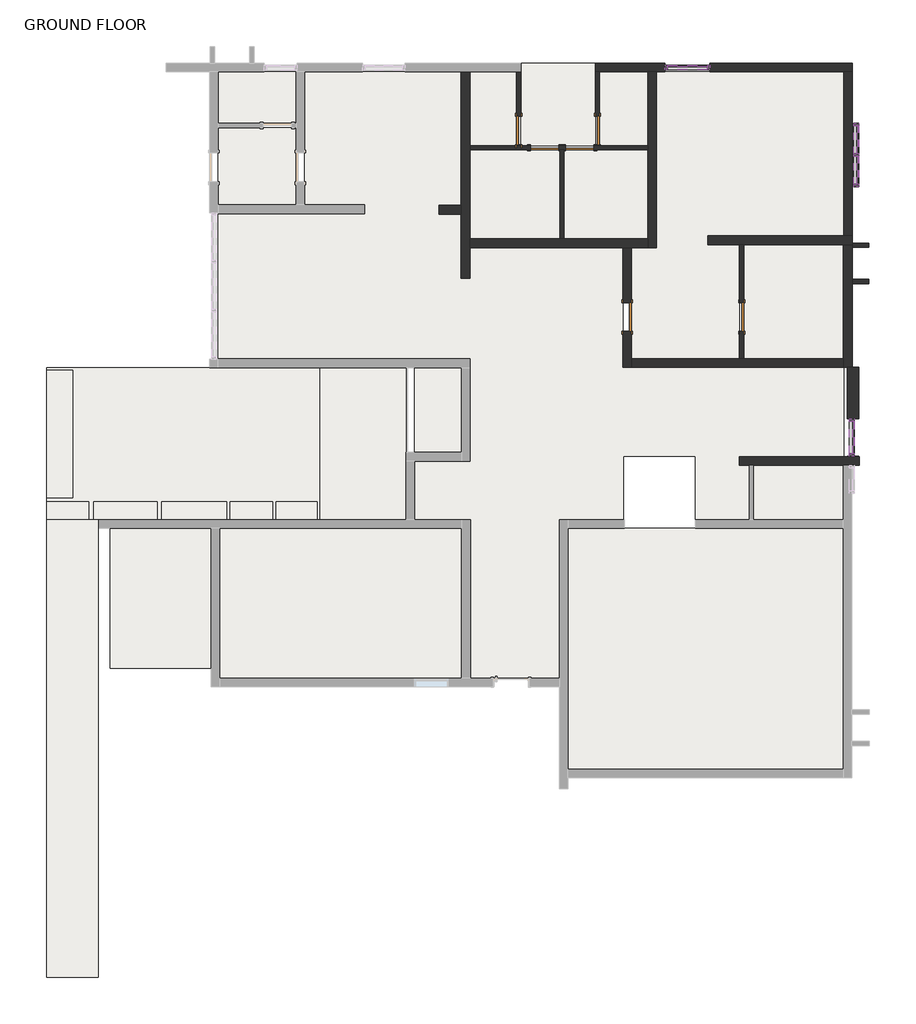
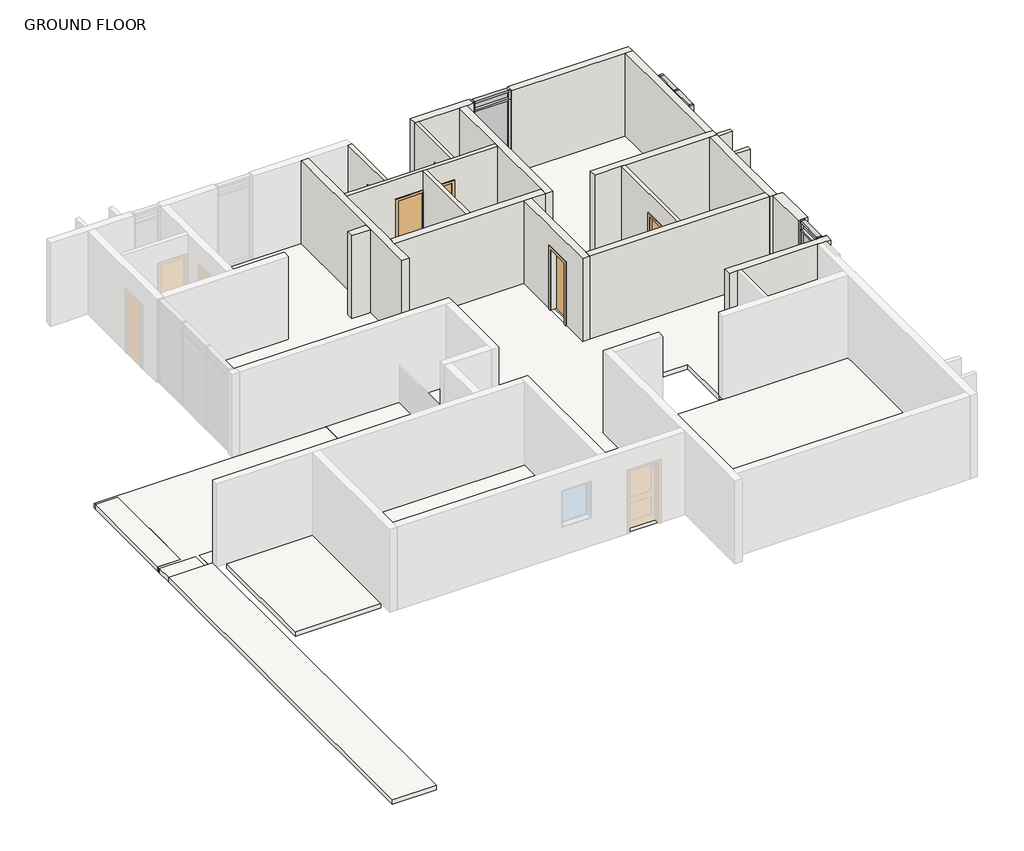
# One storey, part 2 of 2: 26 members, 19 walls, 10 slabs, 8 plates, 6 doors.
"""IFC4 building model written with IfcOpenShell, lengths in millimetres."""

from ifc_helpers import new_model, si_unit, frame, origin, place, context, project, spatial, polyline, outline, extrude, faceted_brep, transform, mapped, element, save
from components import door_d8f5dbb5, door_f2b275c1, door_85036156, member_f0fea5a5, member_75d1e245, member_ee409385, member_3c3dc66a, member_c4de40ee, member_a715cb85, member_3a0a7659, member_7b995701, member_b70ee1cc, member_fd92426f, system_panel_glazed_daed1646, system_panel_glazed_5a33b61e, system_panel_glazed_65d20654, system_panel_glazed_2bc0fbab, system_panel_glazed_828cd182, system_panel_glazed_34f1e917

model = new_model("IFC4")

# Units and contexts
model_context = context("Model", 3, world=origin())
ifc_project = project(units=[si_unit("LENGTHUNIT", "METRE", prefix="MILLI")], contexts=[model_context])

# Site, building, storey
site = spatial("IfcSite", under=ifc_project)
building = spatial("IfcBuilding", under=site)
storey = spatial("IfcBuildingStorey", under=building, Name="GROUND FLOOR", Elevation=304.8)

# Doors
placement = place(None, origin())
door_shape = door_d8f5dbb5(model_context)
element("IfcDoor", 1, ObjectType="Single-Flush : 30\" x 80\"", at=placement, inside=storey, context=model_context, shape_type="MappedRepresentation", body=[
    mapped(door_shape, transform((4206.557821, 14320.99348, 304.8), x_axis=(-1.0, 0.0, 0.0), y_axis=(0.0, -1.0, 0.0), z_axis=(0.0, 0.0, 1.0))),
])
door_2_shape = door_f2b275c1(model_context)
element("IfcDoor", 2, ObjectType="Single-Flush : 30\" x 80\"", at=placement, inside=storey, context=model_context, shape_type="MappedRepresentation", body=[
    mapped(door_2_shape, transform((3281.383965, 14320.99348, 304.8), x_axis=(1.0, 0.0, 0.0), y_axis=(0.0, 1.0, 0.0), z_axis=(0.0, 0.0, 1.0))),
])
element("IfcDoor", 3, ObjectType="Single-Flush : 30\" x 80\"", at=placement, inside=storey, context=model_context, shape_type="MappedRepresentation", body=[
    mapped(door_2_shape, transform((2592.505991, 14778.19348, 304.8), x_axis=(0.0, -1.0, 0.0), y_axis=(1.0, 0.0, 0.0), z_axis=(0.0, 0.0, 1.0))),
])
element("IfcDoor", 4, ObjectType="Single-Flush : 30\" x 80\"", at=placement, inside=storey, context=model_context, shape_type="MappedRepresentation", body=[
    mapped(door_2_shape, transform((4674.531677, 14778.19348, 304.8), x_axis=(0.0, 1.0, 0.0), y_axis=(-1.0, 0.0, 0.0), z_axis=(0.0, 0.0, 1.0))),
])
element("IfcDoor", 5, ObjectType="Single-Flush : 30\" x 80\"", at=placement, inside=storey, context=model_context, shape_type="MappedRepresentation", body=[
    mapped(door_2_shape, transform((8497.231677, 9842.2195632, 304.8), x_axis=(0.0, 1.0, 0.0), y_axis=(-1.0, 0.0, 0.0), z_axis=(0.0, 0.0, 1.0))),
])
door_3_shape = door_85036156(model_context)
element("IfcDoor", 6, ObjectType="Single-Flush : 30\" x 80\"", at=placement, inside=storey, context=model_context, shape_type="MappedRepresentation", body=[
    mapped(door_3_shape, transform((5461.1464182, 9842.2195632, 304.8), x_axis=(0.0, 1.0, 0.0), y_axis=(-1.0, 0.0, 0.0), z_axis=(0.0, 0.0, 1.0))),
])

# Members
member_shape = member_f0fea5a5(model_context)
element("IfcMember", 7, ObjectType="Rectangular Mullion : 2.5\" x 5\" rectangular", at=placement, inside=storey, context=model_context, shape_type="MappedRepresentation", body=[
    mapped(member_shape, transform((11527.7006591, 14134.2124441, 304.8), x_axis=(0.0, -1.0, 0.0), y_axis=(-1.0, 0.0, 0.0), z_axis=(0.0, 0.0, -1.0))),
])
member_2_shape = member_75d1e245(model_context)
element("IfcMember", 8, ObjectType="Rectangular Mullion : 2.5\" x 5\" rectangular", at=placement, inside=storey, context=model_context, shape_type="MappedRepresentation", body=[
    mapped(member_2_shape, transform((11527.7006591, 14134.2124441, 2743.2), x_axis=(0.0, -1.0, 0.0), y_axis=(-1.0, 0.0, 0.0), z_axis=(0.0, 0.0, -1.0))),
])
member_3_shape = member_ee409385(model_context)
element("IfcMember", 9, ObjectType="Rectangular Mullion : 2.5\" x 5\" rectangular", at=placement, inside=storey, context=model_context, shape_type="MappedRepresentation", body=[
    mapped(member_3_shape, transform((7652.681677, 16444.5375339, 304.8), x_axis=(1.0, 0.0, 0.0), y_axis=(0.0, -1.0, 0.0), z_axis=(0.0, 0.0, -1.0))),
])
element("IfcMember", 10, ObjectType="Rectangular Mullion : 2.5\" x 5\" rectangular", at=placement, inside=storey, context=model_context, shape_type="MappedRepresentation", body=[
    mapped(member_3_shape, transform((11527.7006591, 13296.0124441, 304.8), x_axis=(0.0, -1.0, 0.0), y_axis=(-1.0, 0.0, 0.0), z_axis=(0.0, 0.0, -1.0))),
])
element("IfcMember", 11, ObjectType="Rectangular Mullion : 2.5\" x 5\" rectangular", at=placement, inside=storey, context=model_context, shape_type="MappedRepresentation", body=[
    mapped(member_3_shape, transform((11414.0141504, 6159.46982, 304.8), x_axis=(0.0, -1.0, 0.0), y_axis=(-1.0, 0.0, 0.0), z_axis=(0.0, 0.0, -1.0))),
])
member_4_shape = member_3c3dc66a(model_context)
element("IfcMember", 12, ObjectType="Rectangular Mullion : 2.5\" x 5\" rectangular", at=placement, inside=storey, context=model_context, shape_type="MappedRepresentation", body=[
    mapped(member_4_shape, transform((7652.681677, 16444.5375339, 2743.2), x_axis=(1.0, 0.0, 0.0), y_axis=(0.0, -1.0, 0.0), z_axis=(0.0, 0.0, -1.0))),
])
element("IfcMember", 13, ObjectType="Rectangular Mullion : 2.5\" x 5\" rectangular", at=placement, inside=storey, context=model_context, shape_type="MappedRepresentation", body=[
    mapped(member_4_shape, transform((11527.7006591, 13296.0124441, 2743.2), x_axis=(0.0, -1.0, 0.0), y_axis=(-1.0, 0.0, 0.0), z_axis=(0.0, 0.0, -1.0))),
])
element("IfcMember", 14, ObjectType="Rectangular Mullion : 2.5\" x 5\" rectangular", at=placement, inside=storey, context=model_context, shape_type="MappedRepresentation", body=[
    mapped(member_4_shape, transform((11414.0141504, 6159.46982, 2743.2), x_axis=(0.0, -1.0, 0.0), y_axis=(-1.0, 0.0, 0.0), z_axis=(0.0, 0.0, -1.0))),
])
element("IfcMember", 15, ObjectType="Rectangular Mullion : 2.5\" x 5\" rectangular", at=placement, inside=storey, context=model_context, shape_type="MappedRepresentation", body=[
    mapped(member_4_shape, transform((6458.881677, 16444.5375339, 3048.0), x_axis=(-1.0, 0.0, 0.0), y_axis=(0.0, -1.0, 0.0), z_axis=(0.0, 0.0, 1.0))),
])
element("IfcMember", 16, ObjectType="Rectangular Mullion : 2.5\" x 5\" rectangular", at=placement, inside=storey, context=model_context, shape_type="MappedRepresentation", body=[
    mapped(member_4_shape, transform((11527.7006591, 14972.4124441, 3048.0), x_axis=(0.0, 1.0, 0.0), y_axis=(-1.0, 0.0, 0.0), z_axis=(0.0, 0.0, 1.0))),
])
element("IfcMember", 17, ObjectType="Rectangular Mullion : 2.5\" x 5\" rectangular", at=placement, inside=storey, context=model_context, shape_type="MappedRepresentation", body=[
    mapped(member_4_shape, transform((11414.0141504, 7150.06982, 3048.0), x_axis=(0.0, 1.0, 0.0), y_axis=(-1.0, 0.0, 0.0), z_axis=(0.0, 0.0, 1.0))),
])
element("IfcMember", 18, ObjectType="Rectangular Mullion : 2.5\" x 5\" rectangular", at=placement, inside=storey, context=model_context, shape_type="MappedRepresentation", body=[
    mapped(member_3_shape, transform((6458.881677, 16444.5375339, 2743.2), x_axis=(-1.0, 0.0, 0.0), y_axis=(0.0, -1.0, 0.0), z_axis=(0.0, 0.0, 1.0))),
])
element("IfcMember", 19, ObjectType="Rectangular Mullion : 2.5\" x 5\" rectangular", at=placement, inside=storey, context=model_context, shape_type="MappedRepresentation", body=[
    mapped(member_3_shape, transform((11527.7006591, 14972.4124441, 2743.2), x_axis=(0.0, 1.0, 0.0), y_axis=(-1.0, 0.0, 0.0), z_axis=(0.0, 0.0, 1.0))),
])
element("IfcMember", 20, ObjectType="Rectangular Mullion : 2.5\" x 5\" rectangular", at=placement, inside=storey, context=model_context, shape_type="MappedRepresentation", body=[
    mapped(member_3_shape, transform((11414.0141504, 7150.06982, 2743.2), x_axis=(0.0, 1.0, 0.0), y_axis=(-1.0, 0.0, 0.0), z_axis=(0.0, 0.0, 1.0))),
])
member_5_shape = member_c4de40ee(model_context)
element("IfcMember", 21, ObjectType="Rectangular Mullion : 2.5\" x 5\" rectangular", at=placement, inside=storey, context=model_context, shape_type="MappedRepresentation", body=[
    mapped(member_5_shape, transform((7589.181677, 16444.5375339, 3048.0), x_axis=(0.0, 0.0, 1.0), y_axis=(0.0, -1.0, 0.0), z_axis=(1.0, 0.0, 0.0))),
])
element("IfcMember", 22, ObjectType="Rectangular Mullion : 2.5\" x 5\" rectangular", at=placement, inside=storey, context=model_context, shape_type="MappedRepresentation", body=[
    mapped(member_5_shape, transform((6522.381677, 16444.5375339, 304.8), x_axis=(0.0, 0.0, -1.0), y_axis=(0.0, -1.0, 0.0), z_axis=(-1.0, 0.0, 0.0))),
])
member_6_shape = member_a715cb85(model_context)
element("IfcMember", 23, ObjectType="Rectangular Mullion : 2.5\" x 5\" rectangular", at=placement, inside=storey, context=model_context, shape_type="MappedRepresentation", body=[
    mapped(member_6_shape, transform((7589.181677, 16444.5375339, 2743.2), x_axis=(0.0, 0.0, 1.0), y_axis=(0.0, -1.0, 0.0), z_axis=(1.0, 0.0, 0.0))),
])
member_7_shape = member_3a0a7659(model_context)
element("IfcMember", 24, ObjectType="Rectangular Mullion : 2.5\" x 5\" rectangular", at=placement, inside=storey, context=model_context, shape_type="MappedRepresentation", body=[
    mapped(member_7_shape, transform((11527.7006591, 13359.5124441, 3048.0), x_axis=(0.0, 0.0, 1.0), y_axis=(-1.0, 0.0, 0.0), z_axis=(0.0, -1.0, 0.0))),
])
element("IfcMember", 25, ObjectType="Rectangular Mullion : 2.5\" x 5\" rectangular", at=placement, inside=storey, context=model_context, shape_type="MappedRepresentation", body=[
    mapped(member_7_shape, transform((11527.7006591, 14165.9624441, 3048.0), x_axis=(0.0, 0.0, 1.0), y_axis=(-1.0, 0.0, 0.0), z_axis=(0.0, -1.0, 0.0))),
])
element("IfcMember", 26, ObjectType="Rectangular Mullion : 2.5\" x 5\" rectangular", at=placement, inside=storey, context=model_context, shape_type="MappedRepresentation", body=[
    mapped(member_7_shape, transform((11527.7006591, 14908.9124441, 304.8), x_axis=(0.0, 0.0, -1.0), y_axis=(-1.0, 0.0, 0.0), z_axis=(0.0, 1.0, 0.0))),
])
element("IfcMember", 27, ObjectType="Rectangular Mullion : 2.5\" x 5\" rectangular", at=placement, inside=storey, context=model_context, shape_type="MappedRepresentation", body=[
    mapped(member_7_shape, transform((11527.7006591, 14102.4624441, 304.8), x_axis=(0.0, 0.0, -1.0), y_axis=(-1.0, 0.0, 0.0), z_axis=(0.0, 1.0, 0.0))),
])
member_8_shape = member_7b995701(model_context)
element("IfcMember", 28, ObjectType="Rectangular Mullion : 2.5\" x 5\" rectangular", at=placement, inside=storey, context=model_context, shape_type="MappedRepresentation", body=[
    mapped(member_8_shape, transform((11527.7006591, 14165.9624441, 2743.2), x_axis=(0.0, 0.0, 1.0), y_axis=(-1.0, 0.0, 0.0), z_axis=(0.0, -1.0, 0.0))),
])
element("IfcMember", 29, ObjectType="Rectangular Mullion : 2.5\" x 5\" rectangular", at=placement, inside=storey, context=model_context, shape_type="MappedRepresentation", body=[
    mapped(member_8_shape, transform((11527.7006591, 13359.5124441, 2743.2), x_axis=(0.0, 0.0, 1.0), y_axis=(-1.0, 0.0, 0.0), z_axis=(0.0, -1.0, 0.0))),
])
member_9_shape = member_b70ee1cc(model_context)
element("IfcMember", 30, ObjectType="Rectangular Mullion : 2.5\" x 5\" rectangular", at=placement, inside=storey, context=model_context, shape_type="MappedRepresentation", body=[
    mapped(member_9_shape, transform((11414.0141504, 6222.96982, 3048.0), x_axis=(0.0, 0.0, 1.0), y_axis=(-1.0, 0.0, 0.0), z_axis=(0.0, -1.0, 0.0))),
])
element("IfcMember", 31, ObjectType="Rectangular Mullion : 2.5\" x 5\" rectangular", at=placement, inside=storey, context=model_context, shape_type="MappedRepresentation", body=[
    mapped(member_9_shape, transform((11414.0141504, 7086.56982, 304.8), x_axis=(0.0, 0.0, -1.0), y_axis=(-1.0, 0.0, 0.0), z_axis=(0.0, 1.0, 0.0))),
])
member_10_shape = member_fd92426f(model_context)
element("IfcMember", 32, ObjectType="Rectangular Mullion : 2.5\" x 5\" rectangular", at=placement, inside=storey, context=model_context, shape_type="MappedRepresentation", body=[
    mapped(member_10_shape, transform((11414.0141504, 6222.96982, 2743.2), x_axis=(0.0, 0.0, 1.0), y_axis=(-1.0, 0.0, 0.0), z_axis=(0.0, -1.0, 0.0))),
])

# Plates
system_panel_glazed_shape = system_panel_glazed_daed1646(model_context)
element("IfcPlate", 33, ObjectType="System Panel : Glazed", at=placement, inside=storey, context=model_context, shape_type="MappedRepresentation", body=[
    mapped(system_panel_glazed_shape, transform((7055.781677, 16444.5375339, 368.3), x_axis=(1.0, 0.0, 0.0), y_axis=(0.0, 1.0, 0.0), z_axis=(0.0, 0.0, 1.0))),
])
system_panel_glazed_2_shape = system_panel_glazed_5a33b61e(model_context)
element("IfcPlate", 34, ObjectType="System Panel : Glazed", at=placement, inside=storey, context=model_context, shape_type="MappedRepresentation", body=[
    mapped(system_panel_glazed_2_shape, transform((7055.781677, 16444.5375339, 2774.95), x_axis=(1.0, 0.0, 0.0), y_axis=(0.0, 1.0, 0.0), z_axis=(0.0, 0.0, 1.0))),
])
system_panel_glazed_3_shape = system_panel_glazed_65d20654(model_context)
element("IfcPlate", 35, ObjectType="System Panel : Glazed", at=placement, inside=storey, context=model_context, shape_type="MappedRepresentation", body=[
    mapped(system_panel_glazed_3_shape, transform((11527.7006591, 14537.4374441, 368.3), x_axis=(0.0, -1.0, 0.0), y_axis=(1.0, 0.0, 0.0), z_axis=(0.0, 0.0, 1.0))),
])
element("IfcPlate", 36, ObjectType="System Panel : Glazed", at=placement, inside=storey, context=model_context, shape_type="MappedRepresentation", body=[
    mapped(system_panel_glazed_3_shape, transform((11527.7006591, 13730.9874441, 368.3), x_axis=(0.0, -1.0, 0.0), y_axis=(1.0, 0.0, 0.0), z_axis=(0.0, 0.0, 1.0))),
])
system_panel_glazed_4_shape = system_panel_glazed_2bc0fbab(model_context)
element("IfcPlate", 37, ObjectType="System Panel : Glazed", at=placement, inside=storey, context=model_context, shape_type="MappedRepresentation", body=[
    mapped(system_panel_glazed_4_shape, transform((11527.7006591, 14537.4374441, 2774.95), x_axis=(0.0, -1.0, 0.0), y_axis=(1.0, 0.0, 0.0), z_axis=(0.0, 0.0, 1.0))),
])
element("IfcPlate", 38, ObjectType="System Panel : Glazed", at=placement, inside=storey, context=model_context, shape_type="MappedRepresentation", body=[
    mapped(system_panel_glazed_4_shape, transform((11527.7006591, 13730.9874441, 2774.95), x_axis=(0.0, -1.0, 0.0), y_axis=(1.0, 0.0, 0.0), z_axis=(0.0, 0.0, 1.0))),
])
system_panel_glazed_5_shape = system_panel_glazed_828cd182(model_context)
element("IfcPlate", 39, ObjectType="System Panel : Glazed", at=placement, inside=storey, context=model_context, shape_type="MappedRepresentation", body=[
    mapped(system_panel_glazed_5_shape, transform((11414.0141504, 6654.76982, 368.3), x_axis=(0.0, -1.0, 0.0), y_axis=(1.0, 0.0, 0.0), z_axis=(0.0, 0.0, 1.0))),
])
system_panel_glazed_6_shape = system_panel_glazed_34f1e917(model_context)
element("IfcPlate", 40, ObjectType="System Panel : Glazed", at=placement, inside=storey, context=model_context, shape_type="MappedRepresentation", body=[
    mapped(system_panel_glazed_6_shape, transform((11414.0141504, 6654.76982, 2774.95), x_axis=(0.0, -1.0, 0.0), y_axis=(1.0, 0.0, 0.0), z_axis=(0.0, 0.0, 1.0))),
])

# Slabs
element("IfcSlab", 41, ObjectType="FLOORING 6\"", at=placement, inside=storey, context=model_context, shape_type="SweptSolid", body=[
    extrude(outline(polyline([(-3306.644009, 16327.59348), (-3306.644009, 14968.69348), (-5364.044009, 14968.69348), (-5364.044009, 16327.59348), (-3306.644009, 16327.59348)])), frame((0.0, 0.0, 152.4), z_axis=(0.0, 0.0, 1.0), x_axis=(1.0, 0.0, 0.0)), (0.0, 0.0, 1.0), 152.4),
    extrude(outline(polyline([(-3306.644009, 14854.39348), (-3306.644009, 12808.8097639), (-5364.044009, 12808.8097639), (-5364.044009, 14854.39348), (-3306.644009, 14854.39348)])), frame((0.0, 0.0, 152.4), z_axis=(0.0, 0.0, 1.0), x_axis=(1.0, 0.0, 0.0)), (0.0, 0.0, 1.0), 152.4),
    extrude(outline(polyline([(3795.733965, 11907.99348), (3795.733965, 14263.84348), (6014.381677, 14263.84348), (6014.381677, 11907.99348), (3795.733965, 11907.99348)])), frame((0.0, 0.0, 152.4), z_axis=(0.0, 0.0, 1.0), x_axis=(1.0, 0.0, 0.0)), (0.0, 0.0, 1.0), 152.4),
    extrude(outline(polyline([(1297.105991, 11907.99348), (1297.105991, 14263.84348), (3681.433965, 14263.84348), (3681.433965, 11907.99348), (1297.105991, 11907.99348)])), frame((0.0, 0.0, 152.4), z_axis=(0.0, 0.0, 1.0), x_axis=(1.0, 0.0, 0.0)), (0.0, 0.0, 1.0), 152.4),
    extrude(outline(polyline([(8554.381677, 11758.2375339), (11191.5415524, 11758.2375339), (11191.5415524, 8737.3195632), (8554.381677, 8737.3195632), (8554.381677, 11758.2375339)])), frame((0.0, 0.0, 152.4), z_axis=(0.0, 0.0, 1.0), x_axis=(1.0, 0.0, 0.0)), (0.0, 0.0, 1.0), 152.4),
    extrude(outline(polyline([(1080.6237558, 4247.6216143), (1080.6237558, 285.2216143), (-5326.5262442, 285.2216143), (-5326.5262442, 4247.6216143), (1080.6237558, 4247.6216143)])), frame((0.0, 0.0, 152.4), z_axis=(0.0, 0.0, 1.0), x_axis=(1.0, 0.0, 0.0)), (0.0, 0.0, 1.0), 152.4),
    extrude(outline(polyline([(3897.2367729, -2119.417542), (3897.2367729, 4249.632458), (11185.4141504, 4249.632458), (11185.4141504, -2119.417542), (3897.2367729, -2119.417542)])), frame((0.0, 0.0, 152.4), z_axis=(0.0, 0.0, 1.0), x_axis=(1.0, 0.0, 0.0)), (0.0, 0.0, 1.0), 152.4),
    extrude(outline(polyline([(3668.6367729, 285.2216143), (1309.2237558, 285.2216143), (1309.2237558, 4476.2216143), (-167.6931047, 4476.2216143), (-167.6931047, 6029.6356247), (1305.5068953, 6029.6356247), (1305.5068953, 8734.7356247), (-5364.044009, 8734.7356247), (-5364.044009, 12580.2097639), (-1493.8979576, 12580.2097639), (-1493.8979576, 12808.8097639), (-3078.044009, 12808.8097639), (-3078.044009, 16327.59348), (1068.505991, 16327.59348), (1068.505991, 12796.99348), (484.305991, 12796.99348), (484.305991, 12568.39348), (1068.505991, 12568.39348), (1068.505991, 10866.59348), (1297.105991, 10866.59348), (1297.105991, 11679.39348), (5346.8464182, 11679.39348), (5346.8464182, 8508.7195632), (11198.9862453, 8508.7195632), (11198.9862453, 6146.76982), (8430.3862453, 6146.76982), (8430.3862453, 5918.16982), (8696.2141504, 5918.16982), (8696.2141504, 4478.232458), (7273.8141504, 4478.232458), (7273.8141504, 6160.982458), (5364.0867729, 6160.982458), (5364.0867729, 4478.232458), (3668.6367729, 4478.232458), (3668.6367729, 285.2216143)])), frame((0.0, 0.0, 152.4), z_axis=(0.0, 0.0, 1.0), x_axis=(1.0, 0.0, 0.0)), (0.0, 0.0, 1.0), 152.4),
])
element("IfcSlab", 42, ObjectType="FLOORING 6\"", at=placement, inside=storey, context=model_context, shape_type="SweptSolid", body=[
    extrude(outline(polyline([(8440.081677, 8737.3195632), (5575.4464182, 8737.3195632), (5575.4464182, 11679.39348), (6242.981677, 11679.39348), (6242.981677, 16330.2375339), (11195.981677, 16330.2375339), (11195.981677, 11986.8375339), (7601.881677, 11986.8375339), (7601.881677, 11758.2375339), (8440.081677, 11758.2375339), (8440.081677, 8737.3195632)])), frame((0.0, 0.0, 152.4), z_axis=(0.0, 0.0, 1.0), x_axis=(1.0, 0.0, 0.0)), (0.0, 0.0, 1.0), 152.4),
])
element("IfcSlab", 43, ObjectType="MARBLE FLOORING 6\"", at=placement, inside=storey, context=model_context, shape_type="SweptSolid", body=[
    extrude(outline(polyline([(2535.355991, 16327.59348), (2535.355991, 14378.14348), (1297.105991, 14378.14348), (1297.105991, 16327.59348), (2535.355991, 16327.59348)])), frame((0.0, 0.0, 152.4), z_axis=(0.0, 0.0, 1.0), x_axis=(1.0, 0.0, 0.0)), (0.0, 0.0, 1.0), 152.4),
    extrude(outline(polyline([(6014.381677, 16330.2375339), (6014.381677, 14378.14348), (4731.681677, 14378.14348), (4731.681677, 16330.2375339), (6014.381677, 16330.2375339)])), frame((0.0, 0.0, 152.4), z_axis=(0.0, 0.0, 1.0), x_axis=(1.0, 0.0, 0.0)), (0.0, 0.0, 1.0), 152.4),
    extrude(outline(polyline([(4617.381677, 16556.19348), (4617.381677, 14378.14348), (2649.655991, 14378.14348), (2649.655991, 16556.19348), (4617.381677, 16556.19348)])), frame((0.0, 0.0, 152.4), z_axis=(0.0, 0.0, 1.0), x_axis=(1.0, 0.0, 0.0)), (0.0, 0.0, 1.0), 152.4),
])
element("IfcSlab", 44, ObjectType="MARBLE FLOORING 6\"", at=placement, inside=storey, context=model_context, shape_type="SweptSolid", body=[
    extrude(outline(polyline([(-5555.1262442, 4247.6216143), (-5555.1262442, 546.496878), (-8228.4762442, 546.496878), (-8228.4762442, 4247.6216143), (-5555.1262442, 4247.6216143)])), frame((0.0, 0.0, 152.4), z_axis=(0.0, 0.0, 1.0), x_axis=(1.0, 0.0, 0.0)), (0.0, 0.0, 1.0), 152.4),
])
element("IfcSlab", 45, ObjectType="MARBLE FLOORING 6\"", at=placement, inside=storey, context=model_context, shape_type="SweptSolid", body=[
    extrude(outline(polyline([(11185.4141504, 5918.16982), (11185.4141504, 4478.232458), (8810.5141504, 4478.232458), (8810.5141504, 5918.16982), (11185.4141504, 5918.16982)])), frame((0.0, 0.0, 152.4), z_axis=(0.0, 0.0, 1.0), x_axis=(1.0, 0.0, 0.0)), (0.0, 0.0, 1.0), 152.4),
])
element("IfcSlab", 46, ObjectType="MARBLE FLOORING 6\"", at=placement, inside=storey, context=model_context, shape_type="SweptSolid", body=[
    extrude(outline(polyline([(1076.9068953, 8506.1356247), (1076.9068953, 6258.2356247), (-167.6931047, 6258.2356247), (-167.6931047, 8506.1356247), (1076.9068953, 8506.1356247)])), frame((0.0, 0.0, 152.4), z_axis=(0.0, 0.0, 1.0), x_axis=(1.0, 0.0, 0.0)), (0.0, 0.0, 1.0), 152.4),
])
element("IfcSlab", 47, ObjectType="SITE FLOORING 6\"", at=placement, inside=storey, context=model_context, shape_type="SweptSolid", body=[
    extrude(outline(polyline([(-396.2931047, 8506.1356247), (-396.2931047, 4476.2216143), (-2675.406008, 4476.2216143), (-2675.406008, 8506.1356247), (-396.2931047, 8506.1356247)])), frame((0.0, 0.0, 152.4), z_axis=(0.0, 0.0, 1.0), x_axis=(1.0, 0.0, 0.0)), (0.0, 0.0, 1.0), 152.4),
])
element("IfcSlab", 48, ObjectType="SITE FLOORING 6\"", at=placement, inside=storey, context=model_context, shape_type="SweptSolid", body=[
    extrude(outline(polyline([(-2675.406008, 4476.2216143), (-2735.5381686, 4476.2216143), (-2735.5381686, 4971.5216143), (-3840.4381686, 4971.5216143), (-3840.4381686, 4476.2216143), (-3916.6381686, 4476.2216143), (-3916.6381686, 4971.5216143), (-5059.6381686, 4971.5216143), (-5059.6381686, 4476.2216143), (-5135.8381686, 4476.2216143), (-5135.8381686, 4971.5216143), (-6882.0881686, 4971.5216143), (-6882.0881686, 4476.2216143), (-6970.9881686, 4476.2216143), (-6970.9881686, 4971.5216143), (-8679.1381686, 4971.5216143), (-8679.1381686, 4476.2216143), (-8780.7381686, 4476.2216143), (-8780.7381686, 4971.5216143), (-9911.9908689, 4971.5216143), (-9911.9908689, 5047.7216143), (-9200.7908689, 5047.7216143), (-9200.7908689, 8451.3216143), (-9911.9908689, 8451.3216143), (-9911.9908689, 8504.39348), (-2675.406008, 8504.39348), (-2675.406008, 4476.2216143)])), frame((0.0, 0.0, 152.4), z_axis=(0.0, 0.0, 1.0), x_axis=(1.0, 0.0, 0.0)), (0.0, 0.0, 1.0), 152.4),
])
element("IfcSlab", 49, ObjectType="SITE FLOORING 6\"", at=placement, inside=storey, context=model_context, shape_type="SweptSolid", body=[
    extrude(outline(polyline([(-3840.4381686, 4971.5216143), (-2735.5381686, 4971.5216143), (-2735.5381686, 4476.2216143), (-3840.4381686, 4476.2216143), (-3840.4381686, 4971.5216143)])), frame((0.0, 0.0, 152.4), z_axis=(0.0, 0.0, 1.0), x_axis=(1.0, 0.0, 0.0)), (0.0, 0.0, 1.0), 152.4),
    extrude(outline(polyline([(-3916.6381686, 4971.5216143), (-3916.6381686, 4476.2216143), (-5059.6381686, 4476.2216143), (-5059.6381686, 4971.5216143), (-3916.6381686, 4971.5216143)])), frame((0.0, 0.0, 152.4), z_axis=(0.0, 0.0, 1.0), x_axis=(1.0, 0.0, 0.0)), (0.0, 0.0, 1.0), 152.4),
    extrude(outline(polyline([(-5135.8381686, 4971.5216143), (-5135.8381686, 4476.2216143), (-6882.0881686, 4476.2216143), (-6882.0881686, 4971.5216143), (-5135.8381686, 4971.5216143)])), frame((0.0, 0.0, 152.4), z_axis=(0.0, 0.0, 1.0), x_axis=(1.0, 0.0, 0.0)), (0.0, 0.0, 1.0), 152.4),
    extrude(outline(polyline([(-6970.9881686, 4971.5216143), (-6970.9881686, 4476.2216143), (-8679.1381686, 4476.2216143), (-8679.1381686, 4971.5216143), (-6970.9881686, 4971.5216143)])), frame((0.0, 0.0, 152.4), z_axis=(0.0, 0.0, 1.0), x_axis=(1.0, 0.0, 0.0)), (0.0, 0.0, 1.0), 152.4),
    extrude(outline(polyline([(-8780.7381686, 4971.5216143), (-8780.7381686, 4476.2216143), (-9911.9908689, 4476.2216143), (-9911.9908689, 4971.5216143), (-8780.7381686, 4971.5216143)])), frame((0.0, 0.0, 152.4), z_axis=(0.0, 0.0, 1.0), x_axis=(1.0, 0.0, 0.0)), (0.0, 0.0, 1.0), 152.4),
    extrude(outline(polyline([(-9200.7908689, 8451.3216143), (-9200.7908689, 5047.7216143), (-9911.9908689, 5047.7216143), (-9911.9908689, 8451.3216143), (-9200.7908689, 8451.3216143)])), frame((0.0, 0.0, 152.4), z_axis=(0.0, 0.0, 1.0), x_axis=(1.0, 0.0, 0.0)), (0.0, 0.0, 1.0), 152.4),
])
element("IfcSlab", 50, ObjectType="SITE FLOORING 6\"", at=placement, inside=storey, context=model_context, shape_type="SweptSolid", body=[
    extrude(outline(polyline([(-8539.6262442, 4476.2216143), (-8539.6262442, -7636.0724221), (-9911.9908689, -7636.0724221), (-9911.9908689, 4476.2216143), (-8539.6262442, 4476.2216143)])), frame((0.0, 0.0, 152.4), z_axis=(0.0, 0.0, 1.0), x_axis=(1.0, 0.0, 0.0)), (0.0, 0.0, 1.0), 152.4),
])

# Walls
element("IfcWall", 51, ObjectType="INNER WALL 4.5\"", at=placement, inside=storey, context=model_context, shape_type="SweptSolid", body=[
    extrude(outline(polyline([(3795.733965, 14263.84348), (3795.733965, 11907.99348), (3681.433965, 11907.99348), (3681.433965, 14263.84348), (3795.733965, 14263.84348)])), frame((0.0, 0.0, 304.8), z_axis=(0.0, 0.0, 1.0), x_axis=(1.0, 0.0, 0.0)), (0.0, 0.0, 1.0), 2743.2),
])
element("IfcWall", 52, ObjectType="INNER WALL 4.5\"", at=placement, inside=storey, context=model_context, shape_type="Brep", body=[
    faceted_brep([(3662.383965, 14263.84348, 2336.8), (3662.383965, 14263.84348, 304.8), (3681.433965, 14263.84348, 304.8), (3795.733965, 14263.84348, 304.8), (3825.557821, 14263.84348, 304.8), (3825.557821, 14263.84348, 2336.8), (4587.557821, 14263.84348, 2336.8), (4587.557821, 14263.84348, 304.8), (6014.381677, 14263.84348, 304.8), (6014.381677, 14263.84348, 3048.0), (3795.733965, 14263.84348, 3048.0), (3681.433965, 14263.84348, 3048.0), (1297.105991, 14263.84348, 3048.0), (1297.105991, 14263.84348, 304.8), (2900.383965, 14263.84348, 304.8), (2900.383965, 14263.84348, 2336.8), (3825.557821, 14378.14348, 304.8), (3662.383965, 14378.14348, 304.8), (3662.383965, 14378.14348, 2336.8), (2900.383965, 14378.14348, 2336.8), (2900.383965, 14378.14348, 304.8), (2649.655991, 14378.14348, 304.8), (2535.355991, 14378.14348, 304.8), (1297.105991, 14378.14348, 304.8), (1297.105991, 14378.14348, 3048.0), (2535.355991, 14378.14348, 3048.0), (2649.655991, 14378.14348, 3048.0), (4617.381677, 14378.14348, 3048.0), (4731.681677, 14378.14348, 3048.0), (6014.381677, 14378.14348, 3048.0), (6014.381677, 14378.14348, 304.8), (4731.681677, 14378.14348, 304.8), (4617.381677, 14378.14348, 304.8), (4587.557821, 14378.14348, 304.8), (4587.557821, 14378.14348, 2336.8), (3825.557821, 14378.14348, 2336.8)], [[[0, 1, 2, 3, 4, 5, 6, 7, 8, 9, 10, 11, 12, 13, 14, 15]], [[16, 17, 18, 19, 20, 21, 22, 23, 24, 25, 26, 27, 28, 29, 30, 31, 32, 33, 34, 35]], [[33, 32, 31, 30, 8, 7]], [[14, 13, 23, 22, 21, 20]], [[4, 3, 2, 1, 17, 16]], [[12, 11, 10, 9, 29, 28, 27, 26, 25, 24]], [[9, 8, 30, 29]], [[13, 12, 24, 23]], [[5, 4, 16, 35]], [[6, 5, 35, 34]], [[7, 6, 34, 33]], [[18, 17, 1, 0]], [[19, 18, 0, 15]], [[20, 19, 15, 14]]]),
])
element("IfcWall", 53, ObjectType="INNER WALL 4.5\"", at=placement, inside=storey, context=model_context, shape_type="SweptSolid", body=[
    extrude(outline(polyline([(14397.19348, 2336.8), (14397.19348, 304.8), (14378.14348, 304.8), (14378.14348, 3048.0), (16327.59348, 3048.0), (16327.59348, 304.8), (15159.19348, 304.8), (15159.19348, 2336.8), (14397.19348, 2336.8)])), frame((2535.355991, 0.0, 0.0), z_axis=(1.0, 0.0, 0.0), x_axis=(0.0, 1.0, 0.0)), (0.0, 0.0, 1.0), 114.3),
])
element("IfcWall", 54, ObjectType="INNER WALL 4.5\"", at=placement, inside=storey, context=model_context, shape_type="SweptSolid", body=[
    extrude(outline(polyline([(16330.2375339, 304.8), (15159.19348, 304.8), (15159.19348, 2336.8), (14397.19348, 2336.8), (14397.19348, 304.8), (14378.14348, 304.8), (14378.14348, 3048.0), (16330.2375339, 3048.0), (16330.2375339, 304.8)])), frame((4617.381677, 0.0, 0.0), z_axis=(1.0, 0.0, 0.0), x_axis=(0.0, 1.0, 0.0)), (0.0, 0.0, 1.0), 114.3),
])
element("IfcWall", 55, ObjectType="INNER WALL 4.5\"", at=placement, inside=storey, context=model_context, shape_type="SweptSolid", body=[
    extrude(outline(polyline([(11758.2375339, 304.8), (10223.2195632, 304.8), (10223.2195632, 2336.8), (9461.2195632, 2336.8), (9461.2195632, 304.8), (8737.3195632, 304.8), (8737.3195632, 3048.0), (11758.2375339, 3048.0), (11758.2375339, 304.8)])), frame((8440.081677, 0.0, 0.0), z_axis=(1.0, 0.0, 0.0), x_axis=(0.0, 1.0, 0.0)), (0.0, 0.0, 1.0), 114.3),
])
element("IfcWall", 56, ObjectType="INNER WALL 4.5\"", at=placement, inside=storey, context=model_context, shape_type="SweptSolid", body=[
    extrude(outline(polyline([(11424.581677, 11801.3225685), (11861.2634761, 11801.3225685), (11861.2634761, 11687.0225685), (11420.1415524, 11687.0225685), (11420.1415524, 11758.2375339), (11424.581677, 11758.2375339), (11424.581677, 11801.3225685)])), frame((0.0, 0.0, 304.8), z_axis=(0.0, 0.0, 1.0), x_axis=(1.0, 0.0, 0.0)), (0.0, 0.0, 1.0), 2743.2),
])
element("IfcWall", 57, ObjectType="INNER WALL 4.5\"", at=placement, inside=storey, context=model_context, shape_type="SweptSolid", body=[
    extrude(outline(polyline([(11861.2634761, 10726.1319106), (11420.1415524, 10726.1319106), (11420.1415524, 10840.4319106), (11861.2634761, 10840.4319106), (11861.2634761, 10726.1319106)])), frame((0.0, 0.0, 304.8), z_axis=(0.0, 0.0, 1.0), x_axis=(1.0, 0.0, 0.0)), (0.0, 0.0, 1.0), 2743.2),
])
element("IfcWall", 58, ObjectType="OUTER WALL THICKNESS 9\"", at=placement, inside=storey, context=model_context, shape_type="Brep", body=[
    faceted_brep([(11424.581677, 16330.2375339, 304.8), (11424.581677, 16330.2375339, 3048.0), (11195.981677, 16330.2375339, 3048.0), (7652.681677, 16330.2375339, 3048.0), (7652.681677, 16330.2375339, 304.8), (11195.981677, 16330.2375339, 304.8), (11424.581677, 16558.8375339, 3048.0), (11424.581677, 16558.8375339, 304.8), (7652.681677, 16558.8375339, 304.8), (7652.681677, 16558.8375339, 3048.0)], [[[0, 1, 2, 3, 4, 5]], [[6, 7, 8, 9]], [[7, 0, 5, 4, 8]], [[1, 6, 9, 3, 2]], [[1, 0, 7, 6]], [[4, 3, 9, 8]]]),
    faceted_brep([(4617.381677, 16330.2375339, 3048.0), (4617.381677, 16330.2375339, 304.8), (4731.681677, 16330.2375339, 304.8), (6014.381677, 16330.2375339, 304.8), (6242.981677, 16330.2375339, 304.8), (6458.881677, 16330.2375339, 304.8), (6458.881677, 16330.2375339, 3048.0), (6242.981677, 16330.2375339, 3048.0), (6014.381677, 16330.2375339, 3048.0), (4731.681677, 16330.2375339, 3048.0), (4617.381677, 16558.8375339, 304.8), (4617.381677, 16558.8375339, 3048.0), (6458.881677, 16558.8375339, 3048.0), (6458.881677, 16558.8375339, 304.8)], [[[0, 1, 2, 3, 4, 5, 6, 7, 8, 9]], [[10, 11, 12, 13]], [[1, 10, 13, 5, 4, 3, 2]], [[11, 0, 9, 8, 7, 6, 12]], [[1, 0, 11, 10]], [[6, 5, 13, 12]]]),
])
element("IfcWall", 59, ObjectType="OUTER WALL THICKNESS 9\"", at=placement, inside=storey, context=model_context, shape_type="SweptSolid", body=[
    extrude(outline(polyline([(11195.981677, 11986.8375339), (11195.981677, 16330.2375339), (11424.581677, 16330.2375339), (11424.581677, 11986.8375339), (11195.981677, 11986.8375339)])), frame((0.0, 0.0, 304.8), z_axis=(0.0, 0.0, 1.0), x_axis=(1.0, 0.0, 0.0)), (0.0, 0.0, 1.0), 2743.2),
])
element("IfcWall", 60, ObjectType="OUTER WALL THICKNESS 9\"", at=placement, inside=storey, context=model_context, shape_type="Brep", body=[
    faceted_brep([(11424.581677, 11986.8375339, 304.8), (11195.981677, 11986.8375339, 304.8), (7601.881677, 11986.8375339, 304.8), (7601.881677, 11986.8375339, 3048.0), (11195.981677, 11986.8375339, 3048.0), (11424.581677, 11986.8375339, 3048.0), (11424.581677, 11758.2375339, 304.8), (11424.581677, 11758.2375339, 3048.0), (11420.1415524, 11758.2375339, 3048.0), (11191.5415524, 11758.2375339, 3048.0), (8554.381677, 11758.2375339, 3048.0), (8440.081677, 11758.2375339, 3048.0), (7601.881677, 11758.2375339, 3048.0), (7601.881677, 11758.2375339, 304.8), (8440.081677, 11758.2375339, 304.8), (8554.381677, 11758.2375339, 304.8), (11191.5415524, 11758.2375339, 304.8), (11420.1415524, 11758.2375339, 304.8), (11424.581677, 11801.3225685, 304.8), (11424.581677, 11801.3225685, 3048.0)], [[[0, 1, 2, 3, 4, 5]], [[6, 7, 8, 9, 10, 11, 12, 13, 14, 15, 16, 17]], [[2, 1, 0, 18, 6, 17, 16, 15, 14, 13]], [[3, 2, 13, 12]], [[5, 4, 3, 12, 11, 10, 9, 8, 7, 19]], [[0, 5, 19, 7, 6, 18]]]),
])
element("IfcWall", 61, ObjectType="OUTER WALL THICKNESS 9\"", at=placement, inside=storey, context=model_context, shape_type="Brep", body=[
    faceted_brep([(6242.981677, 11679.39348, 304.8), (6242.981677, 16330.2375339, 304.8), (6242.981677, 16330.2375339, 3048.0), (6242.981677, 11679.39348, 3048.0), (6014.381677, 11679.39348, 304.8), (6014.381677, 11679.39348, 3048.0), (6014.381677, 11907.99348, 3048.0), (6014.381677, 14263.84348, 3048.0), (6014.381677, 14378.14348, 3048.0), (6014.381677, 16330.2375339, 3048.0), (6014.381677, 16330.2375339, 304.8), (6014.381677, 14378.14348, 304.8), (6014.381677, 14263.84348, 304.8), (6014.381677, 11907.99348, 304.8)], [[[0, 1, 2, 3]], [[4, 5, 6, 7, 8, 9, 10, 11, 12, 13]], [[1, 0, 4, 13, 12, 11, 10]], [[3, 2, 9, 8, 7, 6, 5]], [[2, 1, 10, 9]], [[0, 3, 5, 4]]]),
])
element("IfcWall", 62, ObjectType="OUTER WALL THICKNESS 9\"", at=placement, inside=storey, context=model_context, shape_type="Brep", body=[
    faceted_brep([(1068.505991, 16327.59348, 304.8), (1068.505991, 12796.99348, 304.8), (1068.505991, 12568.39348, 304.8), (1068.505991, 10866.59348, 304.8), (1068.505991, 10866.59348, 3048.0), (1068.505991, 12568.39348, 3048.0), (1068.505991, 12796.99348, 3048.0), (1068.505991, 16327.59348, 3048.0), (1297.105991, 16327.59348, 304.8), (1297.105991, 16327.59348, 3048.0), (1297.105991, 14378.14348, 3048.0), (1297.105991, 14263.84348, 3048.0), (1297.105991, 11907.99348, 3048.0), (1297.105991, 11679.39348, 3048.0), (1297.105991, 10866.59348, 3048.0), (1297.105991, 10866.59348, 304.8), (1297.105991, 11679.39348, 304.8), (1297.105991, 11907.99348, 304.8), (1297.105991, 14263.84348, 304.8), (1297.105991, 14378.14348, 304.8)], [[[0, 1, 2, 3, 4, 5, 6, 7]], [[8, 9, 10, 11, 12, 13, 14, 15, 16, 17, 18, 19]], [[3, 2, 1, 0, 8, 19, 18, 17, 16, 15]], [[4, 3, 15, 14]], [[7, 6, 5, 4, 14, 13, 12, 11, 10, 9]], [[0, 7, 9, 8]]]),
])
element("IfcWall", 63, ObjectType="OUTER WALL THICKNESS 9\"", at=placement, inside=storey, context=model_context, shape_type="SweptSolid", body=[
    extrude(outline(polyline([(484.305991, 12796.99348), (1068.505991, 12796.99348), (1068.505991, 12568.39348), (484.305991, 12568.39348), (484.305991, 12796.99348)])), frame((0.0, 0.0, 304.8), z_axis=(0.0, 0.0, 1.0), x_axis=(1.0, 0.0, 0.0)), (0.0, 0.0, 1.0), 2743.2),
])
element("IfcWall", 64, ObjectType="OUTER WALL THICKNESS 9\"", at=placement, inside=storey, context=model_context, shape_type="Brep", body=[
    faceted_brep([(11420.1415524, 8508.7195632, 304.8), (11420.1415524, 10726.1319106, 304.8), (11420.1415524, 10840.4319106, 304.8), (11420.1415524, 11687.0225685, 304.8), (11420.1415524, 11758.2375339, 304.8), (11420.1415524, 11758.2375339, 3048.0), (11420.1415524, 11687.0225685, 3048.0), (11420.1415524, 10840.4319106, 3048.0), (11420.1415524, 10726.1319106, 3048.0), (11420.1415524, 8508.7195632, 3048.0), (11191.5415524, 8508.7195632, 304.8), (11191.5415524, 8508.7195632, 3048.0), (11191.5415524, 8737.3195632, 3048.0), (11191.5415524, 11758.2375339, 3048.0), (11191.5415524, 11758.2375339, 304.8), (11191.5415524, 8737.3195632, 304.8), (11293.7494205, 8508.7195632, 304.8), (11293.7494205, 8508.7195632, 3048.0)], [[[0, 1, 2, 3, 4, 5, 6, 7, 8, 9]], [[10, 11, 12, 13, 14, 15]], [[4, 3, 2, 1, 0, 16, 10, 15, 14]], [[9, 8, 7, 6, 5, 13, 12, 11, 17]], [[5, 4, 14, 13]], [[0, 9, 17, 11, 10, 16]]]),
])
element("IfcWall", 65, ObjectType="OUTER WALL THICKNESS 9\"", at=placement, inside=storey, context=model_context, shape_type="Brep", body=[
    faceted_brep([(5346.8464182, 11679.39348, 304.8), (5346.8464182, 10223.2195632, 304.8), (5346.8464182, 10223.2195632, 2336.8), (5346.8464182, 9461.2195632, 2336.8), (5346.8464182, 9461.2195632, 304.8), (5346.8464182, 8508.7195632, 304.8), (5346.8464182, 8508.7195632, 3048.0), (5346.8464182, 11679.39348, 3048.0), (5575.4464182, 10223.2195632, 2336.8), (5575.4464182, 10223.2195632, 304.8), (5575.4464182, 11679.39348, 304.8), (5575.4464182, 11679.39348, 3048.0), (5575.4464182, 8737.3195632, 3048.0), (5575.4464182, 8508.7195632, 3048.0), (5575.4464182, 8508.7195632, 304.8), (5575.4464182, 8737.3195632, 304.8), (5575.4464182, 9461.2195632, 304.8), (5575.4464182, 9461.2195632, 2336.8)], [[[0, 1, 2, 3, 4, 5, 6, 7]], [[8, 9, 10, 11, 12, 13, 14, 15, 16, 17]], [[10, 9, 1, 0]], [[16, 15, 14, 5, 4]], [[7, 6, 13, 12, 11]], [[6, 5, 14, 13]], [[0, 7, 11, 10]], [[2, 1, 9, 8]], [[3, 2, 8, 17]], [[4, 3, 17, 16]]]),
])
element("IfcWall", 66, ObjectType="OUTER WALL THICKNESS 9\"", at=placement, inside=storey, context=model_context, shape_type="Brep", body=[
    faceted_brep([(5575.4464182, 8508.7195632, 304.8), (11191.5415524, 8508.7195632, 304.8), (11191.5415524, 8508.7195632, 3048.0), (5575.4464182, 8508.7195632, 3048.0), (5575.4464182, 8737.3195632, 304.8), (5575.4464182, 8737.3195632, 3048.0), (8440.081677, 8737.3195632, 3048.0), (8554.381677, 8737.3195632, 3048.0), (11191.5415524, 8737.3195632, 3048.0), (11191.5415524, 8737.3195632, 304.8), (8554.381677, 8737.3195632, 304.8), (8440.081677, 8737.3195632, 304.8)], [[[0, 1, 2, 3]], [[4, 5, 6, 7, 8, 9, 10, 11]], [[1, 0, 4, 11, 10, 9]], [[3, 2, 8, 7, 6, 5]], [[2, 1, 9, 8]], [[0, 3, 5, 4]]]),
])
element("IfcWall", 67, ObjectType="OUTER WALL THICKNESS 9\"", at=placement, inside=storey, context=model_context, shape_type="Brep", body=[
    faceted_brep([(1297.105991, 11679.39348, 304.8), (5346.8464182, 11679.39348, 304.8), (5575.4464182, 11679.39348, 304.8), (6014.381677, 11679.39348, 304.8), (6014.381677, 11679.39348, 3048.0), (5575.4464182, 11679.39348, 3048.0), (5346.8464182, 11679.39348, 3048.0), (1297.105991, 11679.39348, 3048.0), (1297.105991, 11907.99348, 304.8), (1297.105991, 11907.99348, 3048.0), (3681.433965, 11907.99348, 3048.0), (3795.733965, 11907.99348, 3048.0), (6014.381677, 11907.99348, 3048.0), (6014.381677, 11907.99348, 304.8), (3795.733965, 11907.99348, 304.8), (3681.433965, 11907.99348, 304.8)], [[[0, 1, 2, 3, 4, 5, 6, 7]], [[8, 9, 10, 11, 12, 13, 14, 15]], [[3, 2, 1, 0, 8, 15, 14, 13]], [[7, 6, 5, 4, 12, 11, 10, 9]], [[4, 3, 13, 12]], [[0, 7, 9, 8]]]),
])
element("IfcWall", 68, ObjectType="OUTER WALL THICKNESS 9\"", at=placement, inside=storey, context=model_context, shape_type="Brep", body=[
    faceted_brep([(11605.3862453, 6146.76982, 304.8), (11598.5494205, 6146.76982, 304.8), (11293.7494205, 6146.76982, 304.8), (8430.3862453, 6146.76982, 304.8), (8430.3862453, 6146.76982, 3048.0), (11293.7494205, 6146.76982, 3048.0), (11598.5494205, 6146.76982, 3048.0), (11605.3862453, 6146.76982, 3048.0), (11605.3862453, 5918.16982, 304.8), (11605.3862453, 5918.16982, 3048.0), (11414.0141504, 5918.16982, 3048.0), (11185.4141504, 5918.16982, 3048.0), (8810.5141504, 5918.16982, 3048.0), (8696.2141504, 5918.16982, 3048.0), (8430.3862453, 5918.16982, 3048.0), (8430.3862453, 5918.16982, 304.8), (8696.2141504, 5918.16982, 304.8), (8810.5141504, 5918.16982, 304.8), (11185.4141504, 5918.16982, 304.8), (11414.0141504, 5918.16982, 304.8)], [[[0, 1, 2, 3, 4, 5, 6, 7]], [[8, 9, 10, 11, 12, 13, 14, 15, 16, 17, 18, 19]], [[3, 2, 1, 0, 8, 19, 18, 17, 16, 15]], [[4, 3, 15, 14]], [[7, 6, 5, 4, 14, 13, 12, 11, 10, 9]], [[0, 7, 9, 8]]]),
])
element("IfcWall", 69, ObjectType="WALL THICKNESS 1'", at=placement, inside=storey, context=model_context, shape_type="Brep", body=[
    faceted_brep([(11293.7494205, 8508.7195632, 3048.0), (11293.7494205, 8508.7195632, 304.8), (11293.7494205, 7150.06982, 304.8), (11293.7494205, 7150.06982, 3048.0), (11598.5494205, 8508.7195632, 304.8), (11598.5494205, 8508.7195632, 3048.0), (11598.5494205, 7150.06982, 3048.0), (11598.5494205, 7150.06982, 304.8), (11420.1415524, 8508.7195632, 304.8), (11420.1415524, 8508.7195632, 3048.0)], [[[0, 1, 2, 3]], [[4, 5, 6, 7]], [[1, 8, 4, 7, 2]], [[5, 9, 0, 3, 6]], [[1, 0, 9, 5, 4, 8]], [[3, 2, 7, 6]]]),
    faceted_brep([(11293.7494205, 6146.76982, 304.8), (11293.7494205, 6146.76982, 3048.0), (11293.7494205, 6159.46982, 3048.0), (11293.7494205, 6159.46982, 304.8), (11598.5494205, 6146.76982, 3048.0), (11598.5494205, 6146.76982, 304.8), (11598.5494205, 6159.46982, 304.8), (11598.5494205, 6159.46982, 3048.0)], [[[0, 1, 2, 3]], [[4, 5, 6, 7]], [[5, 0, 3, 6]], [[1, 4, 7, 2]], [[1, 0, 5, 4]], [[3, 2, 7, 6]]]),
])

save(model, "model.ifc")

# Revit data of these elements
# Type "Single-Flush : 30\" x 80\""
#   Type Mark = "5"
#   Construction Type Id = "MDOOR"
#   Assembly Code = "C1020"
#   Analytic Construction = "Metal"
#   Thickness = 0' - 2"
#   Heat Transfer Coefficient (U) = 0.651978 BTU/(h·ft²·°F)
#   Height = 6' - 8"
#   Trim Projection Ext = 0' - 1"
#   Trim Projection Int = 0' - 1"
#   Trim Width = 0' - 3"
#   Width = 2' - 6"
#   Define Thermal Properties by = 1
#   Define Thermal Properties by = 1
#   Door Material = Door - Panel
#   Frame Material = Door - Frame
#   Visual Light Transmittance = 0
#   Solar Heat Gain Coefficient = 0
#   Function = (empty or 0)
#   Wall Closure = (empty or 0)
# Type "Rectangular Mullion : 2.5\" x 5\" rectangular"
#   built-in parameter 1007304 = 0.416667 (stored number, unit not read)
#   built-in parameter 1007301 = 0.104167 (stored number, unit not read)
#   built-in parameter 1007300 = 0.104167 (stored number, unit not read)
# Type "System Panel : Glazed"
#   Construction Type Id = "GSP4R"
#   Analytic Construction = "1/8 in Pilkington single glazing"
#   Visual Light Transmittance = 0.9
#   Solar Heat Gain Coefficient = 0.86
#   Heat Transfer Coefficient (U) = 1.18115 BTU/(h·ft²·°F)
#   Define Thermal Properties by = 1
# Type "FLOORING 6\""
#   Assembly Code = "B1010"
#   Function = 0
#   Layers, outside or top first: 0' - 6" "MARBLE FLOORING 6\"" (function 1)
# Type "MARBLE FLOORING 6\""
#   Assembly Code = "B1010"
#   Function = 0
#   Layers, outside or top first: 0' - 6" "TILES FLOORING 6\"" (function 1)
# Type "SITE FLOORING 6\""
#   Assembly Code = "B1010"
#   Function = 0
#   Layers, outside or top first: 0' - 6" "SITE FLOORING" (function 1)
# Type "INNER WALL 4.5\""
#   Assembly Code = "B2010"
#   Layers, outside or top first: 0' - 4 1/2" "BEIGE COLOUR" (function 1)
# Type "OUTER WALL THICKNESS 9\""
#   Assembly Code = "B2010"
#   Layers, outside or top first: 0' - 9" "BEIGE COLOUR" (function 1)
# Type "WALL THICKNESS 1'"
#   Assembly Code = "B2010"
#   Layers, outside or top first: 1' - 0" "BEIGE COLOUR" (function 1)
# Elements 1, 2, 3, 4, 5, 6 (IfcDoor, "Single-Flush : 30\" x 80\"")
#   Phase Created = New Construction
#   Materials on its faces: "Door - Frame", "Door - Panel"
# Elements 7, 8, 9, 10, 11, 12, 13, 14, 15, 16, 17, 18, 19, 20, 21, 22, 23, 24, 25, 26, 27, 28, 29, 30, 31, 32 (IfcMember, "Rectangular Mullion : 2.5\" x 5\" rectangular")
#   Phase Created = New Construction
#   Materials on its faces: "Aluminum"
# Elements 33, 34, 35, 36, 37, 38, 39, 40 (IfcPlate, "System Panel : Glazed")
#   Phase Created = New Construction
#   Materials on its faces: "Glass"
# Elements 41, 42 (IfcSlab, "FLOORING 6\"")
#   Height Offset From Level = 0' - 0"
#   Phase Created = New Construction
#   Materials on its faces: "MARBLE FLOORING 6\""
# Elements 43, 44, 45, 46 (IfcSlab, "MARBLE FLOORING 6\"")
#   Height Offset From Level = 0' - 0"
#   Phase Created = New Construction
#   Materials on its faces: "TILES FLOORING 6\""
# Elements 47, 50 (IfcSlab, "SITE FLOORING 6\"")
#   Height Offset From Level = 0' - 0"
#   Phase Created = New Construction
#   Materials on its faces: "SITE FLOORING"
# Element 48 (IfcSlab, "SITE FLOORING 6\"")
#   built-in parameter 1001955 = -1.5708 (stored number, unit not read)
#   Height Offset From Level = 0' - 0"
#   Phase Created = New Construction
#   Materials on its faces: "SITE FLOORING"
# Element 49 (IfcSlab, "SITE FLOORING 6\"")
#   built-in parameter 1001955 = 3.14159 (stored number, unit not read)
#   Height Offset From Level = 0' - 0"
#   Phase Created = New Construction
#   Materials on its faces: "SITE FLOORING"
# Elements 51, 52, 53, 54, 55, 56, 57 (IfcWall, "INNER WALL 4.5\"")
#   Top Offset = 0' - 0"
#   Base Offset = 0' - 0"
#   wall height = 9' - 0"
#   Phase Created = New Construction
#   Base Constraint = GROUND FLOOR
#   Top Constraint = FIRST FLOOR
#   Materials on its faces: "BEIGE COLOUR"
# Elements 58, 59, 60, 61, 62, 63, 64, 65, 66, 67, 68 (IfcWall, "OUTER WALL THICKNESS 9\"")
#   Top Offset = 0' - 0"
#   Base Offset = 0' - 0"
#   wall height = 9' - 0"
#   Phase Created = New Construction
#   Base Constraint = GROUND FLOOR
#   Top Constraint = FIRST FLOOR
#   Materials on its faces: "BEIGE COLOUR"
# Element 69 (IfcWall, "WALL THICKNESS 1'")
#   Top Offset = 0' - 0"
#   Base Offset = 0' - 0"
#   wall height = 9' - 0"
#   Phase Created = New Construction
#   Base Constraint = GROUND FLOOR
#   Top Constraint = FIRST FLOOR
#   Materials on its faces: "BEIGE COLOUR"
# Materials
#   "Door - Panel": class "Wood", colour RGB 210 159 95, transparency 0, Cost = 0
#   "Door - Frame": colour RGB 118 70 51, transparency 0, Cost = 0
#   "MARBLE FLOORING 6\"": class "Generic", colour RGB 120 120 120, transparency 0, Cost = 0
#   "TILES FLOORING 6\"": class "Generic", colour RGB 120 120 120, transparency 0, Cost = 0
#   "SITE FLOORING": class "Generic", colour RGB 120 120 120, transparency 0, Cost = 0
#   "BEIGE COLOUR": class "Generic", colour RGB 120 120 120, transparency 0, Cost = 0
#   "Aluminum": class "Metal", colour RGB 247 247 247, transparency 0, Description = "Aluminum 6061", Cost = 0
#   "Glass": class "Glass", colour RGB 0 128 192, transparency 0.75, Description = "Soda Lime Glass", Cost = 0
